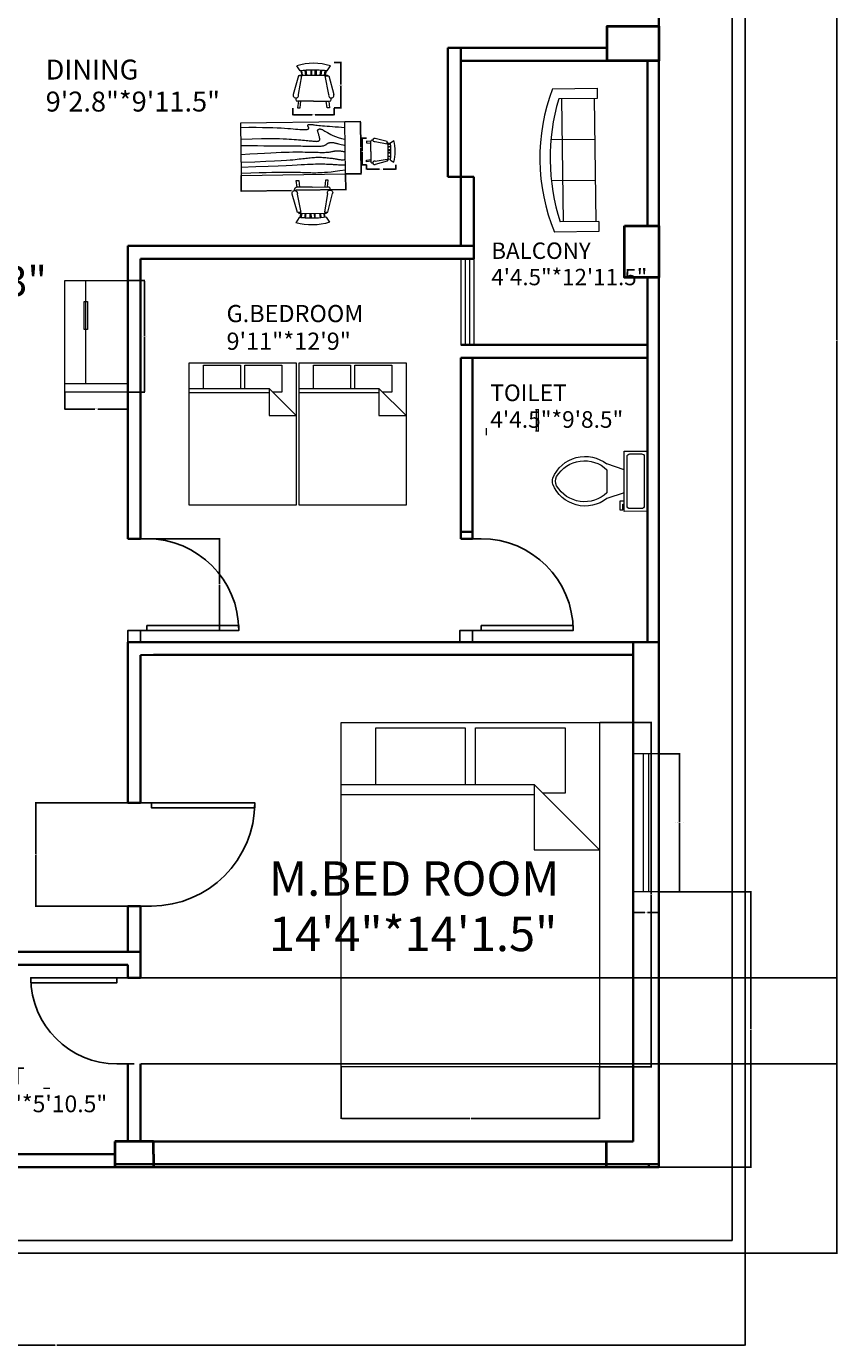
# Model space of a CAD drawing. Units: inches. Extents: x -1085 to 1941, y 1514 to 2348.
# Tile 8 of 9: x 1659 to 1941, y 1514 to 1974. Entities that reach past the tile are written whole.
import ezdxf

# ---------------------------------------------------------------- set-up
doc = ezdxf.new("R2010")
doc.units = ezdxf.units.IN
for name, color, linetype, lineweight in [('A-ANNO-DIMS', 2, 'Continuous', 18), ('A-AREA-IDEN', 7, 'Continuous', 25), ('A-COLS', 7, 'Continuous', 40), ('A-DETL-REFR', 8, 'Continuous', 13), ('A-DOOR', 4, 'Continuous', 25), ('A-EQPM', 9, 'Continuous', 18), ('A-FLOR-FIXT', 9, 'Continuous', 18), ('A-GLAZ', 180, 'Continuous', 18), ('A-WALL', 7, 'Continuous', 35), ('C-PROP', 8, 'Continuous', 25), ('FOUNITR-URE', 2, 'Continuous', 18)]:
    doc.layers.add(name, color=color, linetype=linetype, lineweight=lineweight)
doc.styles.get("Standard").update_dxf_attribs({"font": 'arial.ttf'})
doc.dimstyles.get("Standard").update_dxf_attribs({"dimtxt": 0.18, "dimasz": 0.18, "dimexe": 0.18, "dimexo": 0.0625, "dimgap": 0.09, "dimtad": 0, "dimtih": 1, "dimtoh": 1, "dimdec": 4, "dimzin": 0, "dimdsep": 46, "dimtxsty": 'Standard', "dimcen": 0.09, "dimadec": 0, "dimazin": 0, "dimtfac": 1, "dimtdec": 4, "dimtofl": 0, "dimtmove": 0, "dimatfit": 3, "dimfxl": 1, "dimtolj": 1, "dimtzin": 0, "dimarcsym": 0})

# ---------------------------------------------------------------- blocks, each defined once
blk = doc.blocks.new('*U4')
for p, q in [((0, 0), (0, -6)), ((30, 0), (30, -6))]:
    blk.add_line(p, q)
blk.add_lwpolyline([(0, 0), (0, 30), (1.75, 30), (1.75, 0)], close=True)
blk.add_arc((0, 0), 30, 0, 90)
blk = doc.blocks.new('*U5')
for p, q in [((0, 0), (0, -6)), ((36, 0), (36, -6))]:
    blk.add_line(p, q)
blk.add_lwpolyline([(0, 0), (0, 36), (1.75, 36), (1.75, 0)], close=True)
blk.add_arc((0, 0), 36, 0, 90)
blk = doc.blocks.new('*U3')
for p, q in [((0, 0), (0, -6)), ((32, 0), (32, -6))]:
    blk.add_line(p, q)
blk.add_lwpolyline([(0, 0), (0, 32), (1.75, 32), (1.75, 0)], close=True)
blk.add_arc((0, 0), 32, 0, 90)
blk = doc.blocks.new('Bed - Queen')
for p, q in [((0, -80.00003), (0, 0)), ((0, 0), (59.99999, 0)), ((59.99999, 0), (59.99999, -80.00003)), ((7.99999, -1.2), (28.79998, -1.2)), ((7.99999, -14.4), (7.99999, -1.2)), ((28.79998, -1.2), (28.79998, -14.4)), ((31.19999, -1.2), (51.99999, -1.2)), ((31.19999, -14.4), (31.19999, -1.2)), ((51.99999, -1.2), (51.99999, -16.4)), ((0, -14.4), (44.8, -14.4)), ((59.99999, -29.6), (44.8, -14.4)), ((44.8, -14.4), (44.8, -29.6)), ((44.8, -16.8), (0, -16.8)), ((51.99999, -16.4), (46.79936, -16.4)), ((44.8, -29.6), (59.99999, -29.6)), ((59.99999, -80.00003), (0, -80.00003))]:
    blk.add_line(p, q)
blk = doc.blocks.new('Refrigerator-2 door - 36 in front')
for p, q in [((12, 5), (12, 64)), ((0, 5), (36, 5))]:
    blk.add_line(p, q)
for points in [[(0, 0), (0, 64), (36, 64), (36, 0)], [(11, 36), (11, 52), (13, 52), (13, 36)]]:
    blk.add_lwpolyline(points, close=True)
blk = doc.blocks.new('Toilet - top')
for p, q in [((9.5, -6), (9.5, -2)), ((-10, -8.5), (-8, -8.5)), ((-10, -9.5), (-10, -8.5)), ((-8, -8.5), (-8, -8)), ((-7, -8), (-7, -9.5)), ((-4, -8), (-6, -14)), ((4, -8), (6, -14)), ((-7, -9.5), (-10, -9.5)), ((4, -14), (-4, -14))]:
    blk.add_line(p, q)
blk.add_lwpolyline([(10.5, -8), (10.5, 0), (-10.5, 0), (-10.5, -8)], close=True)
for points in [[(-9.5, -2), (-9.5, -6)], [(8.5, -1), (-8.5, -1)], [(-8.5, -7), (8.5, -7)]]:
    blk.add_lwpolyline(points)
for centre, radius, start, end in [((-8.62, -1.88), 0.884, 81.8699, 188.1301), ((8.62, -1.88), 0.884, 351.8699, 98.1301), ((-8.62, -6.12), 0.884, 171.8699, 278.1301), ((8.62, -6.12), 0.884, 261.8699, 8.1301), ((3.52, -21.58), 12.17, 141.4691, 247.9714), ((4.2, -21.82), 11.33, 136.3677, 238.9468), ((-3.52, -21.58), 12.17, 292.0284, 38.5307), ((-4.2, -21.82), 11.33, 301.053, 43.6321), ((0, -27.88), 4, 245.7318, 294.2682), ((0, -29), 4, 254.8605, 285.1395)]:
    blk.add_arc(centre, radius, start, end)
blk = doc.blocks.new('Table - Rectangular Woodgrain 60 x 30 in.')
for p, q in [((0, 0), (0, -30)), ((60, 0), (0, 0)), ((60, -30), (60, 0)), ((0, -30), (60, -30))]:
    blk.add_line(p, q)
for points in [[(0, -2.4), (4.8155, -2.418), (9.0302, -2.4688), (12.709, -2.5477), (15.9167, -2.65), (18.7181, -2.7711), (21.1781, -2.9063), (23.3616, -3.0508), (25.3333, -3.2), (27.1477, -3.3495), (28.8172, -3.4958), (30.3437, -3.636), (31.7291, -3.7667), (32.9756, -3.8849), (34.0849, -3.9875), (35.059, -4.0714), (35.9, -4.1334), (36.6114, -4.1711), (37.2041, -4.1854), (37.6906, -4.1779), (38.0833, -4.15), (38.3948, -4.1034), (38.6375, -4.0396), (38.8239, -3.9602), (38.9666, -3.8667), (39.0764, -3.7608), (39.1573, -3.6448), (39.2116, -3.521), (39.2416, -3.3917), (39.2498, -3.2593), (39.2385, -3.1261), (39.21, -2.9944), (39.1666, -2.8667), (39.111, -2.7447), (39.0468, -2.6281), (38.978, -2.5163), (38.9083, -2.4083), (38.8418, -2.3035), (38.7823, -2.201), (38.7337, -2.1001), (38.7, -2), (38.6844, -1.9003), (38.6875, -1.8021), (38.7094, -1.707), (38.75, -1.6167), (38.8094, -1.5326), (38.8875, -1.4563), (38.9844, -1.3893), (39.1, -1.3333), (39.2351, -1.2896), (39.3937, -1.2583), (39.5804, -1.2396), (39.8, -1.2333), (40.057, -1.2396), (40.3562, -1.2583), (40.7023, -1.2896), (41.1, -1.3333), (41.5547, -1.3895), (42.0755, -1.4573), (42.6721, -1.5361), (43.3542, -1.625), (44.1316, -1.7233), (45.014, -1.8302), (46.0114, -1.9449), (47.1333, -2.0667), (48.3862, -2.1947), (49.7625, -2.3281), (51.2513, -2.4663), (52.8416, -2.6083), (54.5226, -2.7535), (56.2833, -2.9011), (58.1127, -3.0501), (60, -3.2)], [(0, -9.2), (6.5759, -9.0858), (11.9385, -9.0365), (16.2527, -9.0418), (19.6833, -9.0917), (22.3952, -9.1759), (24.5531, -9.2844), (26.322, -9.4069), (27.8666, -9.5333), (29.3241, -9.6553), (30.7203, -9.7719), (32.0532, -9.8837), (33.3208, -9.9917), (34.5213, -10.0965), (35.6526, -10.199), (36.7128, -10.2999), (37.7, -10.4), (38.6129, -10.4996), (39.4531, -10.5969), (40.223, -10.6895), (40.925, -10.775), (41.5613, -10.8512), (42.1344, -10.9156), (42.6465, -10.966), (43.1, -11), (43.4976, -11.0158), (43.8437, -11.0136), (44.143, -10.9942), (44.4, -10.9583), (44.6195, -10.9069), (44.8062, -10.8406), (44.9648, -10.7603), (45.1, -10.6667), (45.2155, -10.5598), (45.3114, -10.4365), (45.3871, -10.2929), (45.4416, -10.125), (45.4743, -9.929), (45.4844, -9.7011), (45.4709, -9.4371), (45.4333, -9.1333), (45.3716, -8.7883), (45.2896, -8.4104), (45.1919, -8.0107), (45.0833, -7.6), (44.9685, -7.1893), (44.8521, -6.7896), (44.7388, -6.4117), (44.6333, -6.0667), (44.54, -5.7628), (44.4614, -5.4979), (44.4001, -5.2675), (44.3583, -5.0667), (44.3384, -4.8909), (44.3427, -4.7354), (44.3736, -4.5956), (44.4333, -4.4667), (44.5236, -4.3453), (44.6427, -4.2333), (44.7884, -4.1339), (44.9583, -4.05), (45.1501, -3.9849), (45.3614, -3.9417), (45.59, -3.9234), (45.8333, -3.9333), (46.0915, -3.9749), (46.3734, -4.0531), (46.6906, -4.1736), (47.0542, -4.3417), (47.4756, -4.5629), (47.9661, -4.8427), (48.5372, -5.1866), (49.2, -5.6), (49.9676, -6.0844), (50.8594, -6.625), (51.8965, -7.2031), (53.1, -7.8), (54.491, -8.3969), (56.0906, -8.975), (57.9199, -9.5156), (60, -10)], [(0, -12.8), (5.1847, -12.9322), (9.6213, -13.0323), (13.3963, -13.1059), (16.5958, -13.1583), (19.3063, -13.1952), (21.614, -13.2219), (23.6054, -13.2439), (25.3666, -13.2667), (26.9728, -13.2947), (28.4531, -13.3281), (29.8256, -13.3663), (31.1083, -13.4083), (32.3191, -13.4535), (33.476, -13.501), (34.597, -13.5501), (35.7, -13.6), (36.7984, -13.6497), (37.8875, -13.6979), (38.9578, -13.743), (40, -13.7833), (41.0047, -13.8174), (41.9625, -13.8438), (42.864, -13.8607), (43.7, -13.8667), (44.4631, -13.8604), (45.1552, -13.8417), (45.7801, -13.8104), (46.3416, -13.7667), (46.8439, -13.7104), (47.2906, -13.6417), (47.6858, -13.5604), (48.0333, -13.4667), (48.3375, -13.3608), (48.6042, -13.2448), (48.8396, -13.121), (49.05, -12.9917), (49.2417, -12.8593), (49.4208, -12.7261), (49.5937, -12.5944), (49.7667, -12.4667), (49.9452, -12.3451), (50.1323, -12.2313), (50.3303, -12.1268), (50.5416, -12.0333), (50.7686, -11.9524), (51.0135, -11.8854), (51.2788, -11.8341), (51.5666, -11.8), (51.8785, -11.7843), (52.2116, -11.7865), (52.562, -11.8059), (52.926, -11.8417), (53.2998, -11.8931), (53.6795, -11.9594), (54.0614, -12.0397), (54.4416, -12.1333), (54.8223, -12.2401), (55.2293, -12.3625), (55.6942, -12.5037), (56.2489, -12.6667), (56.9251, -12.8547), (57.7545, -13.0708), (58.7689, -13.3182), (60, -13.6)], [(0, -18), (5.124, -17.7273), (9.6609, -17.5057), (13.6705, -17.3303), (17.2125, -17.1958), (20.3467, -17.0973), (23.1328, -17.0297), (25.6307, -16.9878), (27.9, -16.9667), (29.9928, -16.9617), (31.9302, -16.9703), (33.7254, -16.9907), (35.3917, -17.0208), (36.9423, -17.0588), (38.3906, -17.1026), (39.7499, -17.1503), (41.0333, -17.2), (42.2519, -17.2496), (43.4073, -17.2969), (44.4986, -17.3395), (45.525, -17.375), (46.4858, -17.4012), (47.3802, -17.4156), (48.2074, -17.416), (48.9667, -17.4), (49.6583, -17.3662), (50.2872, -17.3167), (50.8595, -17.2547), (51.3812, -17.1833), (51.8584, -17.1057), (52.2971, -17.025), (52.7034, -16.9443), (53.0833, -16.8667), (53.443, -16.7951), (53.789, -16.7313), (54.128, -16.6768), (54.4666, -16.6334), (54.8115, -16.6024), (55.1693, -16.5854), (55.5465, -16.5841), (55.95, -16.6), (56.3828, -16.6337), (56.8346, -16.6823), (57.2915, -16.7418), (57.7396, -16.8084), (58.165, -16.878), (58.5539, -16.9469), (58.8924, -17.0111), (59.1666, -17.0667), (59.3679, -17.1107), (59.5078, -17.1438), (59.6032, -17.1675), (59.6708, -17.1833), (59.7275, -17.193), (59.7901, -17.1979), (59.8753, -17.1998), (60, -17.2)], [(0, -22.4), (8.0098, -22.2501), (14.4094, -22.1011), (19.4168, -21.9535), (23.25, -21.8083), (26.1269, -21.6663), (28.2656, -21.5281), (29.884, -21.3947), (31.2, -21.2667), (32.3967, -21.1448), (33.5172, -21.0292), (34.5697, -20.9198), (35.5625, -20.8167), (36.5037, -20.7198), (37.4015, -20.6292), (38.2642, -20.5448), (39.1, -20.4667), (39.9164, -20.3951), (40.7187, -20.3313), (41.5117, -20.2768), (42.3, -20.2333), (43.0883, -20.2024), (43.8812, -20.1854), (44.6836, -20.1841), (45.5, -20.2), (46.3328, -20.234), (47.1747, -20.2844), (48.0163, -20.3488), (48.8479, -20.425), (49.66, -20.5106), (50.4429, -20.6031), (51.1872, -20.7004), (51.8833, -20.8), (52.5246, -20.8999), (53.1166, -20.9995), (53.6681, -21.0983), (54.1875, -21.1958), (54.6834, -21.2919), (55.1646, -21.3859), (55.6394, -21.4777), (56.1167, -21.5667), (56.6028, -21.6515), (57.0961, -21.7266), (57.5929, -21.7852), (58.0896, -21.8208), (58.5823, -21.8268), (59.0674, -21.7964), (59.5412, -21.723), (60, -21.6)], [(0, -25.2), (8.6355, -25.0504), (15.7026, -24.9031), (21.4049, -24.7606), (25.9458, -24.625), (29.529, -24.4988), (32.3578, -24.3844), (34.6359, -24.284), (36.5667, -24.2), (38.3213, -24.1341), (39.9417, -24.0854), (41.437, -24.0523), (42.8167, -24.0333), (44.0901, -24.0268), (45.2667, -24.0313), (46.3557, -24.0451), (47.3667, -24.0667), (48.309, -24.0947), (49.1928, -24.1287), (50.0284, -24.168), (50.826, -24.2125), (51.5959, -24.2617), (52.3483, -24.3151), (53.0935, -24.3725), (53.8417, -24.4334), (54.6009, -24.497), (55.3699, -24.561), (56.1454, -24.6226), (56.9239, -24.6792), (57.7021, -24.7279), (58.4764, -24.7662), (59.2435, -24.7911), (60, -24.8)], [(0, -28.8), (5.6867, -28.6681), (10.45, -28.5698), (14.407, -28.5012), (17.675, -28.4584), (20.3711, -28.4374), (22.6125, -28.4344), (24.5164, -28.4455), (26.2, -28.4667), (27.762, -28.4947), (29.2276, -28.5281), (30.6033, -28.5663), (31.8958, -28.6084), (33.1118, -28.6535), (34.2578, -28.7011), (35.3405, -28.7501), (36.3666, -28.8), (37.3443, -28.8497), (38.288, -28.8974), (39.2137, -28.9412), (40.1375, -28.9792), (41.0753, -29.0093), (42.0432, -29.0297), (43.0572, -29.0384), (44.1333, -29.0333), (45.2936, -29.0114), (46.5843, -28.9641), (48.0579, -28.8816), (49.7666, -28.7542), (51.7629, -28.5721), (54.0989, -28.3255), (56.8272, -28.0048), (60, -27.6)]]:
    blk.add_lwpolyline(points)
blk = doc.blocks.new('Chair - Rocking')
for p, q in [((-9, -7.5), (-12, -18.49999)), ((-8, -4.5), (-10, -1.5)), ((-7, -7.5), (-9, -7.5)), ((-9, -18.49999), (-7, -7.5)), ((-8.23428, -6.99939), (-8.3093, -7.47958)), ((-8.23041, -7), (8.23915, -7)), ((-7.5, -4.5), (-7, -7)), ((-6.5, -7), (-7.02225, -4.43)), ((-4.5, -7), (-4.96674, -4.19951)), ((-4, -7), (-4.40532, -4.16272)), ((-1.5, -4.05012), (-1.5, -7)), ((-1, -7), (-1, -4.05012)), ((1, -7), (1, -4.04655)), ((1.5, -4.05012), (1.5, -7)), ((4, -7), (4.40187, -4.18694)), ((4.5, -7), (4.96761, -4.19437)), ((6.5, -7), (7, -4.4057)), ((7.5, -4.5), (7, -7)), ((7, -7.5), (9, -7.5)), ((9, -18.49999), (7, -7.5)), ((8, -4.5), (10, -1.5)), ((8.31071, -7.48854), (8.23449, -7.00073)), ((9, -7.5), (12, -18.49999)), ((-10.36644, -20.64523), (-10.5, -21.49999)), ((-9, -22.49999), (-9.5, -26.49999)), ((0, -22.49999), (-9.5, -22.49999)), ((-8, -26.49999), (-7.5, -22.49999)), ((0, -22.49999), (9.5, -22.49999)), ((8, -26.49999), (7.5, -22.49999)), ((9, -22.49999), (9.5, -26.49999)), ((10.5, -21.49999), (10.3575, -20.58798)), ((-9.5, -26.49999), (-8, -26.49999)), ((9.5, -26.49999), (8, -26.49999))]:
    blk.add_line(p, q)
for centre, radius, start, end in [((0, -34.08333), 34.08333, 72.93847, 107.0615), ((0, -68.25004), 64.25, 93.92211, 97.15267), ((0, -68.25004), 64.25, 82.84733, 93.92211), ((-10.5, -18.99999), 1.58114, 161.5651, 18.43495), ((-9.5, -21.49999), 1, 180, 270), ((10.5, -18.99999), 1.58114, 161.5651, 18.43495), ((9.5, -21.49999), 1, 270, 0)]:
    blk.add_arc(centre, radius, start, end)
blk = doc.blocks.new('Sofa - Roundback 7 ft.')
for p, q in [((-12.00002, -32.4421), (-12.00003, -6.5971)), ((11.99997, -32.4421), (11.99998, -6.5971)), ((-36.000027, -34), (-36.000027, -11.4696)), ((-35.999844, -13.3819), (35.9998, -13.3819)), ((35.99998, -34), (35.99998, -11.4696)), ((-36.000027, -32.4421), (35.99998, -32.4421))]:
    blk.add_line(p, q)
for points in [[(-36.000027, -34), (-42.000027, -34), (-42.000027, -8)], [(41.99998, -8), (41.99998, -34), (35.99998, -34)]]:
    blk.add_lwpolyline(points)
for centre, radius, start, end in [((0, -114.25), 114.25, 68.43141, 111.5686), ((-0.00001, -127.1968), 121.1968, 72.72033, 107.2797)]:
    blk.add_arc(centre, radius, start, end)
blk = doc.blocks.new('WIN-48-9')
for p, q in [((9, 48), (0, 48)), ((3.5, 48), (3.5, 0)), ((5.5, 0), (5.5, 48)), ((9, 0), (0, 0))]:
    blk.add_line(p, q)
blk = doc.blocks.new('*D32')
at = {"layer": 'A-ANNO-DIMS', "color": 0, "lineweight": -2, "transparency": 16777216}
for p, q in [((1858.49, 1731.17), (1876.6, 1731.17)), ((1876.42, 1730.99), (1876.42, 1671.37)), ((1876.42, 1611.39), (1876.42, 1671)), ((1858.49, 1611.21), (1876.6, 1611.21))]:
    blk.add_line(p, q, dxfattribs=at)
at = {"layer": 'A-ANNO-DIMS', "color": 0, "transparency": 16777216}
for points in [[(1876.39, 1730.99), (1876.45, 1730.99), (1876.42, 1731.17)], [(1876.39, 1611.39), (1876.45, 1611.39), (1876.42, 1611.21)]]:
    blk.add_solid(points, dxfattribs=at)
at = {"layer": 'Defpoints', "color": 0, "transparency": 16777216}
for p in [(1858.42, 1731.17), (1876.42, 1731.17), (1858.42, 1611.21)]:
    blk.add_point(p, dxfattribs=at)
at = {"layer": 'A-ANNO-DIMS', "color": 0, "transparency": 16777216, "insert": (1876.42, 1671.19), "char_height": 0.18, "attachment_point": 5}
blk.add_mtext('\\A1;BED 120', dxfattribs=at)
blk = doc.blocks.new('*D33')
at = {"layer": 'A-ANNO-DIMS', "color": 0, "lineweight": -2, "transparency": 16777216}
for p, q in [((1768.45, 1611.14), (1768.45, 1593.03)), ((1858.42, 1611.14), (1858.42, 1593.03)), ((1768.63, 1593.21), (1813.22, 1593.21)), ((1858.24, 1593.21), (1813.66, 1593.21))]:
    blk.add_line(p, q, dxfattribs=at)
at = {"layer": 'A-ANNO-DIMS', "color": 0, "transparency": 16777216}
for points in [[(1768.63, 1593.24), (1768.63, 1593.18), (1768.45, 1593.21)], [(1858.24, 1593.24), (1858.24, 1593.18), (1858.42, 1593.21)]]:
    blk.add_solid(points, dxfattribs=at)
at = {"layer": 'Defpoints', "color": 0, "transparency": 16777216}
for p in [(1768.45, 1611.21), (1858.42, 1611.21), (1858.42, 1593.21)]:
    blk.add_point(p, dxfattribs=at)
at = {"layer": 'A-ANNO-DIMS', "color": 0, "transparency": 16777216, "insert": (1813.44, 1593.21), "char_height": 0.18, "attachment_point": 5}
blk.add_mtext('\\A1;90', dxfattribs=at)
blk = doc.blocks.new('*D48')
at = {"layer": 'A-ANNO-DIMS', "color": 0, "lineweight": -2, "transparency": 16777216}
for p, q in [((1733.57, 1921.79), (1733.64, 1916.22)), ((1769.92, 1922.28), (1770, 1916.71)), ((1733.82, 1916.4), (1751.16, 1916.64)), ((1769.81, 1916.89), (1752.47, 1916.66))]:
    blk.add_line(p, q, dxfattribs=at)
at = {"layer": 'A-ANNO-DIMS', "color": 0, "transparency": 16777216}
for points in [[(1733.82, 1916.43), (1733.82, 1916.37), (1733.64, 1916.4)], [(1769.81, 1916.92), (1769.81, 1916.86), (1769.99, 1916.89)]]:
    blk.add_solid(points, dxfattribs=at)
at = {"layer": 'Defpoints', "color": 0, "transparency": 16777216}
for p in [(1733.57, 1921.86), (1769.92, 1922.35), (1769.99, 1916.89)]:
    blk.add_point(p, dxfattribs=at)
at = {"layer": 'A-ANNO-DIMS', "color": 0, "transparency": 16777216, "insert": (1751.82, 1916.65), "char_height": 0.18, "attachment_point": 5}
blk.add_mtext('\\A1;TABLE 36', dxfattribs=at)
blk = doc.blocks.new('*D49')
at = {"layer": 'A-ANNO-DIMS', "color": 0, "lineweight": -2, "transparency": 16777216}
for p, q in [((1769.74, 1940.52), (1775.31, 1940.6)), ((1775.13, 1940.42), (1775.25, 1931.69)), ((1775.37, 1922.6), (1775.25, 1931.33)), ((1769.98, 1922.35), (1775.55, 1922.42))]:
    blk.add_line(p, q, dxfattribs=at)
at = {"layer": 'A-ANNO-DIMS', "color": 0, "transparency": 16777216}
for points in [[(1775.16, 1940.42), (1775.1, 1940.42), (1775.13, 1940.6)], [(1775.4, 1922.6), (1775.34, 1922.6), (1775.37, 1922.42)]]:
    blk.add_solid(points, dxfattribs=at)
at = {"layer": 'Defpoints', "color": 0, "transparency": 16777216}
for p in [(1769.67, 1940.52), (1775.13, 1940.6), (1769.92, 1922.35)]:
    blk.add_point(p, dxfattribs=at)
at = {"layer": 'A-ANNO-DIMS', "color": 0, "transparency": 16777216, "insert": (1775.25, 1931.51), "char_height": 0.18, "attachment_point": 5}
blk.add_mtext('\\A1;18', dxfattribs=at)
blk = doc.blocks.new('*D52')
at = {"layer": 'A-ANNO-DIMS', "color": 0, "lineweight": -2, "transparency": 16777216}
for p, q in [((1766.03, 1961.21), (1768.52, 1961.21)), ((1768.34, 1961.03), (1768.34, 1953.47)), ((1768.34, 1945.55), (1768.34, 1953.1)), ((1766.03, 1945.37), (1768.52, 1945.37))]:
    blk.add_line(p, q, dxfattribs=at)
at = {"layer": 'A-ANNO-DIMS', "color": 0, "transparency": 16777216}
for points in [[(1768.31, 1961.03), (1768.37, 1961.03), (1768.34, 1961.21)], [(1768.31, 1945.55), (1768.37, 1945.55), (1768.34, 1945.37)]]:
    blk.add_solid(points, dxfattribs=at)
at = {"layer": 'Defpoints', "color": 0, "transparency": 16777216}
for p in [(1765.96, 1961.21), (1768.34, 1961.21), (1765.96, 1945.37)]:
    blk.add_point(p, dxfattribs=at)
at = {"layer": 'A-ANNO-DIMS', "color": 0, "transparency": 16777216, "insert": (1768.34, 1953.29), "char_height": 0.18, "attachment_point": 5}
blk.add_mtext('\\A1;CHAIR 16 TYP.', dxfattribs=at)
blk = doc.blocks.new('*D53')
at = {"layer": 'A-ANNO-DIMS', "color": 0, "lineweight": -2, "transparency": 16777216}
for p, q in [((1751.63, 1945.3), (1751.63, 1942.81)), ((1765.96, 1945.3), (1765.96, 1942.81)), ((1751.81, 1942.99), (1758.28, 1942.99)), ((1765.78, 1942.99), (1759.32, 1942.99))]:
    blk.add_line(p, q, dxfattribs=at)
at = {"layer": 'A-ANNO-DIMS', "color": 0, "transparency": 16777216}
for points in [[(1751.81, 1943.02), (1751.81, 1942.96), (1751.63, 1942.99)], [(1765.78, 1943.02), (1765.78, 1942.96), (1765.96, 1942.99)]]:
    blk.add_solid(points, dxfattribs=at)
at = {"layer": 'Defpoints', "color": 0, "transparency": 16777216}
for p in [(1751.63, 1945.37), (1765.96, 1945.37), (1765.96, 1942.99)]:
    blk.add_point(p, dxfattribs=at)
at = {"layer": 'A-ANNO-DIMS', "color": 0, "transparency": 16777216, "insert": (1758.8, 1942.99), "char_height": 0.18, "attachment_point": 5}
blk.add_mtext('\\A1;14 TYP.', dxfattribs=at)
blk = doc.blocks.new('*D54')
at = {"layer": 'A-ANNO-DIMS', "color": 0, "lineweight": -2, "transparency": 16777216}
for p, q in [((1777.25, 1925.51), (1777.25, 1923.86)), ((1777.43, 1924.04), (1781.72, 1924.04)), ((1787.29, 1924.04), (1783, 1924.04)), ((1787.47, 1925.51), (1787.47, 1923.86))]:
    blk.add_line(p, q, dxfattribs=at)
at = {"layer": 'A-ANNO-DIMS', "color": 0, "transparency": 16777216}
for points in [[(1777.43, 1924.07), (1777.43, 1924.01), (1777.25, 1924.04)], [(1787.29, 1924.07), (1787.29, 1924.01), (1787.47, 1924.04)]]:
    blk.add_solid(points, dxfattribs=at)
at = {"layer": 'Defpoints', "color": 0, "transparency": 16777216}
for p in [(1777.25, 1925.57), (1787.47, 1925.57), (1787.47, 1924.04)]:
    blk.add_point(p, dxfattribs=at)
at = {"layer": 'A-ANNO-DIMS', "color": 0, "transparency": 16777216, "insert": (1782.36, 1924.04), "char_height": 0.18, "attachment_point": 5}
blk.add_mtext('\\A1;CHAIR 10', dxfattribs=at)
blk = doc.blocks.new('*D55')
at = {"layer": 'A-ANNO-DIMS', "color": 0, "lineweight": -2, "transparency": 16777216}
for p, q in [((1777.19, 1934.82), (1775.53, 1934.82)), ((1775.71, 1934.64), (1775.71, 1930.38)), ((1775.71, 1925.75), (1775.71, 1930.02)), ((1777.19, 1925.57), (1775.53, 1925.57))]:
    blk.add_line(p, q, dxfattribs=at)
at = {"layer": 'A-ANNO-DIMS', "color": 0, "transparency": 16777216}
for points in [[(1775.68, 1934.64), (1775.74, 1934.64), (1775.71, 1934.82)], [(1775.68, 1925.75), (1775.74, 1925.75), (1775.71, 1925.57)]]:
    blk.add_solid(points, dxfattribs=at)
at = {"layer": 'Defpoints', "color": 0, "transparency": 16777216}
for p in [(1777.25, 1934.82), (1775.71, 1925.57), (1777.25, 1925.57)]:
    blk.add_point(p, dxfattribs=at)
at = {"layer": 'A-ANNO-DIMS', "color": 0, "transparency": 16777216, "insert": (1775.71, 1930.2), "char_height": 0.18, "attachment_point": 5}
blk.add_mtext('\\A1;9', dxfattribs=at)
blk = doc.blocks.new('*D58')
at = {"layer": 'A-ANNO-DIMS', "color": 0, "lineweight": -2, "transparency": 16777216}
for p, q in [((1694.14, 1885.2), (1700.1, 1885.2)), ((1699.92, 1885.02), (1699.92, 1865.92)), ((1699.92, 1846.45), (1699.92, 1865.55)), ((1694.14, 1846.27), (1700.1, 1846.27))]:
    blk.add_line(p, q, dxfattribs=at)
at = {"layer": 'A-ANNO-DIMS', "color": 0, "transparency": 16777216}
for points in [[(1699.89, 1885.02), (1699.95, 1885.02), (1699.92, 1885.2)], [(1699.89, 1846.45), (1699.95, 1846.45), (1699.92, 1846.27)]]:
    blk.add_solid(points, dxfattribs=at)
at = {"layer": 'Defpoints', "color": 0, "transparency": 16777216}
for p in [(1694.08, 1885.2), (1699.92, 1885.2), (1694.08, 1846.27)]:
    blk.add_point(p, dxfattribs=at)
at = {"layer": 'A-ANNO-DIMS', "color": 0, "transparency": 16777216, "insert": (1699.92, 1865.73), "char_height": 0.18, "attachment_point": 5}
blk.add_mtext('\\A1;REFRIGERATOR 39 TYP.', dxfattribs=at)
blk = doc.blocks.new('*D59')
at = {"layer": 'A-ANNO-DIMS', "color": 0, "lineweight": -2, "transparency": 16777216}
for p, q in [((1672.18, 1846.21), (1672.18, 1840.25)), ((1694.08, 1846.21), (1694.08, 1840.25)), ((1672.36, 1840.43), (1682.6, 1840.43)), ((1693.9, 1840.43), (1683.66, 1840.43))]:
    blk.add_line(p, q, dxfattribs=at)
at = {"layer": 'A-ANNO-DIMS', "color": 0, "transparency": 16777216}
for points in [[(1672.36, 1840.46), (1672.36, 1840.4), (1672.18, 1840.43)], [(1693.9, 1840.46), (1693.9, 1840.4), (1694.08, 1840.43)]]:
    blk.add_solid(points, dxfattribs=at)
at = {"layer": 'Defpoints', "color": 0, "transparency": 16777216}
for p in [(1672.18, 1846.27), (1694.08, 1846.27), (1694.08, 1840.43)]:
    blk.add_point(p, dxfattribs=at)
at = {"layer": 'A-ANNO-DIMS', "color": 0, "transparency": 16777216, "insert": (1683.13, 1840.43), "char_height": 0.18, "attachment_point": 5}
blk.add_mtext('\\A1;22 TYP.', dxfattribs=at)
blk = doc.blocks.new('*D68')
at = {"layer": 'A-ANNO-DIMS', "color": 0, "lineweight": -2, "transparency": 16777216}
for p, q in [((1879.16, 1720.24), (1886.47, 1720.24)), ((1886.29, 1720.06), (1886.29, 1696.42)), ((1886.29, 1672.42), (1886.29, 1696.06)), ((1879.16, 1672.24), (1886.47, 1672.24))]:
    blk.add_line(p, q, dxfattribs=at)
at = {"layer": 'A-ANNO-DIMS', "color": 0, "transparency": 16777216}
for points in [[(1886.26, 1720.06), (1886.32, 1720.06), (1886.29, 1720.24)], [(1886.26, 1672.42), (1886.32, 1672.42), (1886.29, 1672.24)]]:
    blk.add_solid(points, dxfattribs=at)
at = {"layer": 'Defpoints', "color": 0, "transparency": 16777216}
for p in [(1879.09, 1720.24), (1886.29, 1720.24), (1879.09, 1672.24)]:
    blk.add_point(p, dxfattribs=at)
at = {"layer": 'A-ANNO-DIMS', "color": 0, "transparency": 16777216, "insert": (1886.29, 1696.24), "char_height": 0.18, "attachment_point": 5}
blk.add_mtext('\\A1;BEDROOM WINDOW 48 TYP.', dxfattribs=at)
blk = doc.blocks.new('*D69')
at = {"layer": 'A-ANNO-DIMS', "color": 0, "lineweight": -2, "transparency": 16777216}
for p, q in [((1870.09, 1672.18), (1870.09, 1664.86)), ((1879.09, 1672.18), (1879.09, 1664.86)), ((1870.27, 1665.04), (1874.14, 1665.04)), ((1878.91, 1665.04), (1875.05, 1665.04))]:
    blk.add_line(p, q, dxfattribs=at)
at = {"layer": 'A-ANNO-DIMS', "color": 0, "transparency": 16777216}
for points in [[(1870.27, 1665.07), (1870.27, 1665.01), (1870.09, 1665.04)], [(1878.91, 1665.07), (1878.91, 1665.01), (1879.09, 1665.04)]]:
    blk.add_solid(points, dxfattribs=at)
at = {"layer": 'Defpoints', "color": 0, "transparency": 16777216}
for p in [(1870.09, 1672.24), (1879.09, 1672.24), (1879.09, 1665.04)]:
    blk.add_point(p, dxfattribs=at)
at = {"layer": 'A-ANNO-DIMS', "color": 0, "transparency": 16777216, "insert": (1874.59, 1665.04), "char_height": 0.18, "attachment_point": 5}
blk.add_mtext('\\A1;9 TYP.', dxfattribs=at)
blk = doc.blocks.new('*D74')
at = {"layer": 'A-ANNO-DIMS', "color": 0, "lineweight": -2, "transparency": 16777216}
for p, q in [((1429.09, 1546.18), (1429.09, 1514.06)), ((1909.09, 1546.18), (1909.09, 1514.06)), ((1429.27, 1514.24), (1668.8, 1514.24)), ((1908.91, 1514.24), (1669.39, 1514.24))]:
    blk.add_line(p, q, dxfattribs=at)
at = {"layer": 'A-ANNO-DIMS', "color": 0, "transparency": 16777216}
for points in [[(1429.27, 1514.27), (1429.27, 1514.21), (1429.09, 1514.24)], [(1908.91, 1514.27), (1908.91, 1514.21), (1909.09, 1514.24)]]:
    blk.add_solid(points, dxfattribs=at)
at = {"layer": 'Defpoints', "color": 0, "transparency": 16777216}
for p in [(1429.09, 1546.24), (1909.09, 1546.24), (1909.09, 1514.24)]:
    blk.add_point(p, dxfattribs=at)
at = {"layer": 'A-ANNO-DIMS', "color": 0, "transparency": 16777216, "insert": (1669.09, 1514.24), "char_height": 0.18, "attachment_point": 5}
blk.add_mtext('\\A1;480', dxfattribs=at)
blk = doc.blocks.new('*D75')
at = {"layer": 'A-ANNO-DIMS', "color": 0, "lineweight": -2, "transparency": 16777216}
for p, q in [((1909.16, 2182.24), (1941.27, 2182.24)), ((1941.09, 2182.06), (1941.09, 1864.42)), ((1941.09, 1546.42), (1941.09, 1864.06)), ((1909.16, 1546.24), (1941.27, 1546.24))]:
    blk.add_line(p, q, dxfattribs=at)
at = {"layer": 'A-ANNO-DIMS', "color": 0, "transparency": 16777216}
for points in [[(1941.06, 2182.06), (1941.12, 2182.06), (1941.09, 2182.24)], [(1941.06, 1546.42), (1941.12, 1546.42), (1941.09, 1546.24)]]:
    blk.add_solid(points, dxfattribs=at)
at = {"layer": 'Defpoints', "color": 0, "transparency": 16777216}
for p in [(1909.09, 2182.24), (1941.09, 2182.24), (1909.09, 1546.24)]:
    blk.add_point(p, dxfattribs=at)
at = {"layer": 'A-ANNO-DIMS', "color": 0, "transparency": 16777216, "insert": (1941.09, 1864.24), "char_height": 0.18, "attachment_point": 5}
blk.add_mtext('\\A1;636', dxfattribs=at)
blk = doc.blocks.new('*D81')
at = {"layer": 'A-ANNO-DIMS', "color": 0, "lineweight": -2, "transparency": 16777216}
for p, q in [((1694.03, 1703.24), (1661.91, 1703.24)), ((1662.09, 1703.06), (1662.09, 1685.42)), ((1662.09, 1667.42), (1662.09, 1685.06)), ((1694.03, 1667.24), (1661.91, 1667.24))]:
    blk.add_line(p, q, dxfattribs=at)
at = {"layer": 'A-ANNO-DIMS', "color": 0, "transparency": 16777216}
for points in [[(1662.06, 1703.06), (1662.12, 1703.06), (1662.09, 1703.24)], [(1662.06, 1667.42), (1662.12, 1667.42), (1662.09, 1667.24)]]:
    blk.add_solid(points, dxfattribs=at)
at = {"layer": 'Defpoints', "color": 0, "transparency": 16777216}
for p in [(1662.09, 1703.24), (1694.09, 1703.24), (1694.09, 1667.24)]:
    blk.add_point(p, dxfattribs=at)
at = {"layer": 'A-ANNO-DIMS', "color": 0, "transparency": 16777216, "insert": (1662.09, 1685.24), "char_height": 0.18, "attachment_point": 5}
blk.add_mtext('\\A1;36', dxfattribs=at)
blk = doc.blocks.new('*D82')
at = {"layer": 'A-ANNO-DIMS', "color": 0, "lineweight": -2, "transparency": 16777216}
for p, q in [((1694.14, 1795.24), (1726.26, 1795.24)), ((1726.08, 1795.06), (1726.08, 1779.42)), ((1726.08, 1763.42), (1726.08, 1779.06)), ((1694.14, 1763.24), (1726.26, 1763.24))]:
    blk.add_line(p, q, dxfattribs=at)
at = {"layer": 'A-ANNO-DIMS', "color": 0, "transparency": 16777216}
for points in [[(1726.05, 1795.06), (1726.11, 1795.06), (1726.08, 1795.24)], [(1726.05, 1763.42), (1726.11, 1763.42), (1726.08, 1763.24)]]:
    blk.add_solid(points, dxfattribs=at)
at = {"layer": 'Defpoints', "color": 0, "transparency": 16777216}
for p in [(1694.08, 1795.24), (1694.08, 1763.24), (1726.08, 1763.24)]:
    blk.add_point(p, dxfattribs=at)
at = {"layer": 'A-ANNO-DIMS', "color": 0, "transparency": 16777216, "insert": (1726.08, 1779.24), "char_height": 0.18, "attachment_point": 5}
blk.add_mtext('\\A1;32', dxfattribs=at)
blk = doc.blocks.new('*D85')
at = {"layer": 'A-ANNO-DIMS', "color": 0, "lineweight": -2, "transparency": 16777216}
for p, q in [((1698.66, 1642.24), (1941.27, 1642.24)), ((1941.09, 1642.06), (1941.09, 1627.42)), ((1941.09, 1612.42), (1941.09, 1627.06)), ((1698.66, 1612.24), (1941.27, 1612.24))]:
    blk.add_line(p, q, dxfattribs=at)
at = {"layer": 'A-ANNO-DIMS', "color": 0, "transparency": 16777216}
for points in [[(1941.06, 1642.06), (1941.12, 1642.06), (1941.09, 1642.24)], [(1941.06, 1612.42), (1941.12, 1612.42), (1941.09, 1612.24)]]:
    blk.add_solid(points, dxfattribs=at)
at = {"layer": 'Defpoints', "color": 0, "transparency": 16777216}
for p in [(1698.59, 1642.24), (1698.59, 1612.24), (1941.09, 1612.24)]:
    blk.add_point(p, dxfattribs=at)
at = {"layer": 'A-ANNO-DIMS', "color": 0, "transparency": 16777216, "insert": (1941.09, 1627.24), "char_height": 0.18, "attachment_point": 5}
blk.add_mtext('\\A1;30', dxfattribs=at)
blk = doc.blocks.new('*D88')
at = {"layer": 'A-ANNO-DIMS', "color": 0, "lineweight": -2, "transparency": 16777216}
for p, q in [((1879.16, 1672.24), (1911.27, 1672.24)), ((1911.09, 1672.06), (1911.09, 1624.42)), ((1911.09, 1576.42), (1911.09, 1624.06)), ((1879.16, 1576.24), (1911.27, 1576.24))]:
    blk.add_line(p, q, dxfattribs=at)
at = {"layer": 'A-ANNO-DIMS', "color": 0, "transparency": 16777216}
for points in [[(1911.06, 1672.06), (1911.12, 1672.06), (1911.09, 1672.24)], [(1911.06, 1576.42), (1911.12, 1576.42), (1911.09, 1576.24)]]:
    blk.add_solid(points, dxfattribs=at)
at = {"layer": 'Defpoints', "color": 0, "transparency": 16777216}
for p in [(1879.09, 1672.24), (1879.09, 1576.24), (1911.09, 1576.24)]:
    blk.add_point(p, dxfattribs=at)
at = {"layer": 'A-ANNO-DIMS', "color": 0, "transparency": 16777216, "insert": (1911.09, 1624.24), "char_height": 0.18, "attachment_point": 5}
blk.add_mtext('\\A1;96', dxfattribs=at)

msp = doc.modelspace()

# ---------------------------------------------------------------- linework, layer by layer
at = {"layer": 'A-COLS'}
for p, q in [((1694.0637, 1585.2392), (1689.5637, 1585.2392)), ((1689.5637, 1585.2392), (1689.5637, 1576.2392)), ((1703.0637, 1585.2392), (1694.0637, 1585.2392)), ((1703.0637, 1580.7392), (1703.0637, 1585.2392)), ((1860.7548, 1585.2392), (1860.7548, 1576.2392)), ((1703.0637, 1580.7392), (1703.0637, 1576.2392))]:
    msp.add_line(p, q, dxfattribs=at)
for points in [[(1879.0949, 1973.8073), (1879.0949, 1961.8073), (1861.0949, 1961.8073), (1861.0949, 1973.8073)], [(1867.0949, 1904.253), (1879.0949, 1904.253), (1879.0949, 1886.253), (1867.0949, 1886.253)]]:
    msp.add_lwpolyline(points, close=True, dxfattribs=at)
at = {"layer": 'A-DETL-REFR'}
for p, q in [((1836.0588, 1840.2288), (1837.3087, 1840.2288)), ((1836.3689, 1840.2288), (1836.3689, 1832.7875)), ((1836.9987, 1840.2288), (1836.9987, 1832.7875)), ((1819.0584, 1831.2883), (1819.0584, 1833.7244)), ((1836.0588, 1832.7875), (1837.3087, 1832.7875)), ((1666.9664, 1603.6946), (1664.7683, 1603.6946))]:
    msp.add_line(p, q, dxfattribs=at)
at = {"layer": 'A-DOOR'}
for points in [[(1698.5793, 1759.2392), (1698.5793, 1760.2392), (1698.5793, 1761.2392), (1698.5793, 1763.2392), (1694.0793, 1763.2392), (1694.0793, 1761.2392), (1694.0793, 1759.2392)], [(1814.2064, 1759.2392), (1814.2064, 1760.2392), (1814.2064, 1761.2392), (1814.2064, 1763.2392), (1809.7064, 1763.2392), (1809.7064, 1761.2392), (1809.7064, 1759.2392)]]:
    msp.add_lwpolyline(points, dxfattribs=at)
at = {"layer": 'A-GLAZ'}
for p, q in [((1810.0793, 1892.7992), (1810.0793, 1862.7992)), ((1811.5793, 1892.7992), (1811.5793, 1862.7992)), ((1813.0793, 1892.7992), (1813.0793, 1862.7992)), ((1814.5793, 1892.7992), (1814.5793, 1862.7992))]:
    msp.add_line(p, q, dxfattribs=at)
at = {"layer": 'A-WALL'}
for p, q in [((1879.0949, 2134.2392), (1879.0949, 1576.2392)), ((1805.5793, 1966.2992), (1861.0949, 1966.2992)), ((1805.5793, 1921.2992), (1805.5793, 1966.2992)), ((1810.0793, 1921.2992), (1810.0793, 1966.2992)), ((1814.5793, 1961.7992), (1810.0793, 1961.7992)), ((1814.5793, 1961.7992), (1875.0637, 1961.7992)), ((1875.0637, 1961.8073), (1875.0637, 1904.253)), ((1814.5793, 1921.2992), (1805.5793, 1921.2992)), ((1810.0793, 1897.2992), (1810.0793, 1921.2992)), ((1814.5793, 1897.2992), (1814.5793, 1921.2992)), ((1694.0793, 1795.2392), (1694.0793, 1897.2992)), ((1694.0793, 1897.2992), (1814.5793, 1897.2992)), ((1814.5793, 1897.2992), (1814.5793, 1892.7992)), ((1698.5793, 1795.2392), (1698.5793, 1892.7992)), ((1698.5793, 1892.7992), (1814.5793, 1892.7992)), ((1875.0637, 1886.253), (1875.0637, 1759.2392)), ((1810.0793, 1862.7992), (1875.0637, 1862.7992)), ((1875.0637, 1864.7816), (1875.0637, 1854.4588)), ((1810.0793, 1858.2992), (1875.0637, 1858.2992)), ((1810.0793, 1858.2992), (1810.0793, 1797.6204)), ((1814.2064, 1797.6204), (1814.2064, 1858.2992)), ((1810.0793, 1797.6204), (1814.2064, 1797.6204)), ((1810.0793, 1797.6204), (1810.0793, 1795.2392)), ((1814.2064, 1797.6204), (1814.2064, 1795.2392)), ((1694.0793, 1795.2392), (1698.5793, 1795.2392)), ((1814.2064, 1795.2392), (1810.0793, 1795.2392)), ((1810.1365, 1795.2392), (1810.1365, 1795.2392)), ((1810.1365, 1795.2392), (1810.1365, 1795.2392)), ((1703.0637, 1759.2392), (1694.0949, 1759.2392)), ((1694.0949, 1703.2392), (1694.0949, 1759.2392)), ((1875.0637, 1759.2392), (1703.0637, 1759.2392)), ((1870.0949, 1759.2392), (1870.0949, 1585.2392)), ((1875.0637, 1759.2392), (1879.0949, 1759.2392)), ((1698.5949, 1754.6644), (1706.7416, 1754.7392)), ((1698.5949, 1703.2392), (1698.5949, 1754.6644)), ((1870.0949, 1754.7392), (1703.0637, 1754.7392)), ((1698.5949, 1703.2392), (1694.0949, 1703.2392)), ((1698.5949, 1667.2392), (1694.0949, 1667.2392)), ((1694.0949, 1667.2392), (1694.0949, 1651.2392)), ((1698.5949, 1642.2392), (1698.5949, 1667.2392)), ((1698.5949, 1651.2392), (1506.0949, 1651.2392)), ((1698.5949, 1642.2392), (1698.5949, 1651.2392)), ((1694.0949, 1646.7392), (1574.5949, 1646.7392)), ((1694.0949, 1642.2392), (1694.0949, 1646.7392)), ((1698.5949, 1642.2392), (1694.0949, 1642.2392)), ((1694.0949, 1585.2392), (1694.0949, 1612.2392)), ((1698.5949, 1585.2392), (1698.5949, 1612.2392)), ((1698.5949, 1585.2392), (1698.5949, 1612.2392)), ((1703.0637, 1585.2392), (1870.0949, 1585.2392)), ((1483.0949, 1580.7392), (1689.5637, 1580.7392)), ((1689.5637, 1577.2392), (1879.0949, 1577.2392)), ((1875.5949, 1577.2392), (1875.5949, 1576.2392)), ((1465.0949, 1576.2392), (1879.0949, 1576.2392))]:
    msp.add_line(p, q, dxfattribs=at)
at = {"layer": 'C-PROP'}
for p, q in [((1909.0949, 2182.2392), (1909.0949, 1546.2392)), ((1904.5949, 2177.7392), (1904.5949, 1550.7392)), ((1433.5949, 1550.7392), (1904.5949, 1550.7392)), ((1429.0949, 1546.2392), (1909.0949, 1546.2392))]:
    msp.add_line(p, q, dxfattribs=at)

# ---------------------------------------------------------------- block references
at = {"layer": 'A-DOOR', "xscale": -1}
for name, p, rotation in [('*U3', (1700.7747, 1763.2392), 270), ('*U3', (1817.2064, 1763.2392), 270), ('*U4', (1690.3449, 1642.2392), 90)]:
    msp.add_blockref(name, p, dxfattribs=dict(at, rotation=rotation))
at = {"layer": 'A-DOOR', "rotation": 270}
msp.add_blockref('*U5', (1702.3449, 1703.2392), dxfattribs=at)
at = {"layer": 'A-EQPM', "xscale": 0.6082930186288423, "yscale": 0.6082930186288423, "zscale": 0.6082930186288423}
msp.add_blockref('Refrigerator-2 door - 36 in front', (1672.1808, 1846.2692), dxfattribs=at)
at = {"layer": 'A-FLOR-FIXT', "xscale": -1, "rotation": 270.0278966559833}
msp.add_blockref('Toilet - top', (1874.9712, 1815.2863), dxfattribs=at)
at = {"layer": 'A-GLAZ'}
msp.add_blockref('WIN-48-9', (1870.095, 1672.239), dxfattribs=at)
at = {"layer": 'FOUNITR-URE'}
for name, p, xscale, yscale, zscale in [('Chair - Rocking', (1758.7966, 1960.9128), 0.586650110807243, 0.586650110807243, 0.586650110807243), ('Bed - Queen', (1715.5429, 1856.497), 0.6202052364975769, 0.6202052364975769, 0.6202052364975769), ('Bed - Queen', (1753.8009, 1856.497), 0.6202052364975769, 0.6202052364975769, 0.6202052364975769), ('Bed - Queen', (1768.4522, 1731.1669), 1.499521534902406, 1.499521534902406, 1.499521534902406)]:
    msp.add_blockref(name, p, dxfattribs=dict(at, xscale=xscale, yscale=yscale, zscale=zscale))
for name, p, xscale, yscale, zscale, rotation in [('Sofa - Roundback 7 ft.', (1837.6181, 1927.0055), 0.5951175733769988, 0.5951175733769988, 0.5951175733769988, 90.70274874306504), ('Table - Rectangular Woodgrain 60 x 30 in.', (1733.3209, 1940.0319), 0.6059375441385758, 0.6059375441385758, 0.6059375441385758, 0.7742742613998593), ('Chair - Rocking', (1787.2843, 1930.1973), 0.3787344361325826, 0.3787344361325826, 0.3787344361325826, 270), ('Chair - Rocking', (1758.5445, 1904.5697), -0.586650110807243, 0.5866501108072432, 0.586650110807243, 180.7908801225163)]:
    msp.add_blockref(name, p, dxfattribs=dict(at, xscale=xscale, yscale=yscale, zscale=zscale, rotation=rotation))

# ---------------------------------------------------------------- texts
at = {"layer": 'A-ANNO-DIMS'}
for s, height, p in [('9\'2.8"*9\'11.5"', 6.94158, (1665.5147, 1944.0988)), ('18\'3.8"*19\'2.3"', 10.510424, (1566.056, 1879.7196)), ('4\'4.5"*12\'11.5"', 5.716045, (1820.7055, 1883.5638)), ('9\'11"*12\'9"', 5.988134, (1728.499, 1861.0832)), ('4\'4.5"*9\'8.5"', 5.794078, (1820.3652, 1833.8919)), ('14\'4"*14\'1.5"', 12, (1743.2936, 1651.5358))]:
    msp.add_text(s, height=height, dxfattribs=at).set_placement(p)
at = {"layer": 'A-AREA-IDEN'}
for s, height, p in [('DINING', 6.94158, (1665.5147, 1955.2499)), ('BALCONY', 5.71605, (1820.7055, 1892.7461)), ('G.BEDROOM', 5.98813, (1728.499, 1870.7027)), ('TOILET', 5.79408, (1820.3652, 1843.1995)), ('M.BED ROOM', 12, (1743.2936, 1670.8128))]:
    msp.add_text(s, height=height, dxfattribs=at).set_placement(p)
at = {"layer": 'A-AREA-IDEN', "insert": (1631.2558, 1611.0202), "char_height": 5.861483, "attachment_point": 1}
msp.add_mtext_dynamic_manual_height_columns('TOILET\\P9\'11.5"*5\'10.5"', width=0.197712, gutter_width=29.3074, heights=[0], dxfattribs=at)

# ---------------------------------------------------------------- dimensions: what is measured, and where the dimension line sits
at = {"layer": 'A-ANNO-DIMS'}
for base, p1, p2, angle, picture, middle in [((1941.0949, 2182.2392), (1909.0949, 1546.2392), (1909.0949, 2182.2392), 90, '*D75', (1941.0949, 1864.2392)), ((1775.1268, 1940.5969), (1769.9195, 1922.3468), (1769.6738, 1940.5232), 90.774274, '*D49', (1775.2496, 1931.5087)), ((1775.714, 1925.5701), (1777.2478, 1934.8245), (1777.2478, 1925.5701), 270, '*D55', (1775.714, 1930.1973)), ((1726.0793, 1763.2392), (1694.0793, 1795.2392), (1694.0793, 1763.2392), 270, '*D82', (1726.0793, 1779.2392)), ((1662.0949, 1703.2392), (1694.0949, 1667.2392), (1694.0949, 1703.2392), 90, '*D81', (1662.0949, 1685.2392)), ((1911.0949, 1576.2392), (1879.0949, 1672.2392), (1879.0949, 1576.2392), 270, '*D88', (1911.0949, 1624.2392)), ((1941.0949, 1612.2392), (1698.5949, 1642.2392), (1698.5949, 1612.2392), 90, '*D85', (1941.0949, 1627.2392))]:
    dim = msp.add_linear_dim(base=base, p1=p1, p2=p2, angle=angle, dimstyle='Standard', override={"dimdec": 0, "dimlfac": 1, "dimrnd": 0, "dimzin": 0, "dimdsep": 46, "dimlunit": 2}, dxfattribs=at)
    dim.commit()
    dim.dimension.update_dxf_attribs({"geometry": picture, "text_midpoint": middle})
for base, p1, p2, angle, text, picture, middle in [((1768.34, 1961.2061), (1765.964, 1945.3665), (1765.964, 1961.2061), 90, 'CHAIR <> TYP.', '*D52', (1768.34, 1953.2863)), ((1769.9932, 1916.8938), (1733.5665, 1921.8555), (1769.9195, 1922.3468), 0.774274, 'TABLE <>', '*D48', (1751.8167, 1916.6482)), ((1699.9189, 1885.2), (1694.0793, 1846.2692), (1694.0793, 1885.2), 90, 'REFRIGERATOR <> TYP.', '*D58', (1699.9189, 1865.7346)), ((1876.4178, 1731.1669), (1858.4235, 1611.2051), (1858.4235, 1731.1669), 90, 'BED <>', '*D32', (1876.4178, 1671.186)), ((1886.2949, 1720.2392), (1879.0949, 1672.2392), (1879.0949, 1720.2392), 90, 'BEDROOM WINDOW <> TYP.', '*D68', (1886.2949, 1696.2392))]:
    dim = msp.add_linear_dim(base=base, p1=p1, p2=p2, angle=angle, text=text, dimstyle='Standard', override={"dimdec": 0, "dimlfac": 1, "dimrnd": 0, "dimzin": 0, "dimdsep": 46, "dimlunit": 2}, dxfattribs=at)
    dim.commit()
    dim.dimension.update_dxf_attribs({"geometry": picture, "text_midpoint": middle})
for base, p1, p2, text, picture, middle in [((1765.964, 1942.9906), (1751.6292, 1945.3665), (1765.964, 1945.3665), '<> TYP.', '*D53', (1758.7966, 1942.9906)), ((1787.4737, 1924.0362), (1777.2478, 1925.5701), (1787.4737, 1925.5701), 'CHAIR <>', '*D54', (1782.3607, 1924.0362)), ((1694.0793, 1840.4296), (1672.1808, 1846.2692), (1694.0793, 1846.2692), '<> TYP.', '*D59', (1683.13, 1840.4296)), ((1879.0949, 1665.0392), (1870.0949, 1672.2392), (1879.0949, 1672.2392), '<> TYP.', '*D69', (1874.5949, 1665.0392))]:
    dim = msp.add_linear_dim(base=base, p1=p1, p2=p2, text=text, dimstyle='Standard', override={"dimdec": 0, "dimlfac": 1, "dimrnd": 0, "dimzin": 0, "dimdsep": 46, "dimlunit": 2}, dxfattribs=at)
    dim.commit()
    dim.dimension.update_dxf_attribs({"geometry": picture, "text_midpoint": middle})
for base, p1, p2, picture, middle in [((1858.4235, 1593.2109), (1768.4522, 1611.2051), (1858.4235, 1611.2051), '*D33', (1813.4379, 1593.2109)), ((1909.0949, 1514.2392), (1429.0949, 1546.2392), (1909.0949, 1546.2392), '*D74', (1669.0949, 1514.2392))]:
    dim = msp.add_linear_dim(base=base, p1=p1, p2=p2, dimstyle='Standard', override={"dimdec": 0, "dimlfac": 1, "dimrnd": 0, "dimzin": 0, "dimdsep": 46, "dimlunit": 2}, dxfattribs=at)
    dim.commit()
    dim.dimension.update_dxf_attribs({"geometry": picture, "text_midpoint": middle})

doc.saveas('drawing.dxf')
